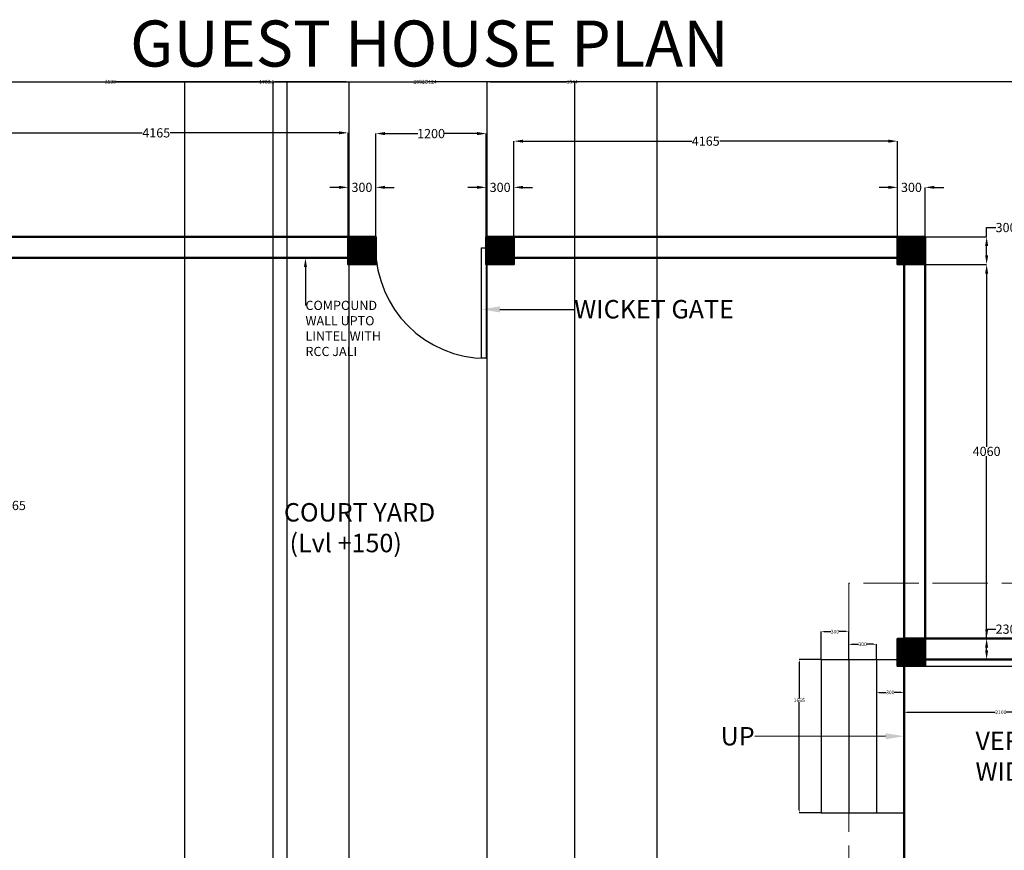
# Model space of a CAD drawing. Units: millimetres. Extents: x -17156 to 39375, y -45872 to -24892.
# Tile 9 of 12: x -5337 to 5351, y -33909 to -24892. Entities that reach past the tile are written whole.
import ezdxf
from ezdxf import colors
from ezdxf.entities.mleader import LeaderData, LeaderLine
from ezdxf.math import Vec2, Vec3

# ---------------------------------------------------------------- set-up
doc = ezdxf.new("R2010")
doc.units = ezdxf.units.MM
doc.header["$MEASUREMENT"] = 0
doc.linetypes.add('ACAD_ISO02W100', pattern=[15, 12, -3])
for name, color, linetype, lineweight in [('A-ANNO-DIMS', 2, 'Continuous', 18), ('A-ANNO-TEXT', 4, 'Continuous', 18), ('A-ANNO-TITL', 4, 'Continuous', 35), ('A-AREA-IDEN', 4, 'Continuous', 25), ('A-COLS', 7, 'Continuous', 40), ('A-ROOF', 8, 'Continuous', 18), ('A-ROOF-OVHD', 8, 'ACAD_ISO02W100', 18), ('DOORS', 6, 'Continuous', 25), ('STEPS', 2, 'Continuous', 25), ('WALLS', 5, 'Continuous', 50)]:
    doc.layers.add(name, color=color, linetype=linetype, lineweight=lineweight)
doc.styles.get("Standard").update_dxf_attribs({"font": 'arial.ttf'})
doc.dimstyles.get("Standard").update_dxf_attribs({"dimtxt": 40, "dimasz": 30.18, "dimexe": 0, "dimexo": 0.0625, "dimgap": 0.09, "dimtad": 0, "dimtih": 1, "dimtoh": 1, "dimdec": 0, "dimzin": 0, "dimdsep": 46, "dimtxsty": 'Standard', "dimcen": 0.09, "dimadec": 0, "dimazin": 0, "dimtfac": 1, "dimtdec": 0, "dimtofl": 0, "dimtmove": 0, "dimatfit": 3, "dimfxl": 1, "dimtolj": 1, "dimtzin": 0, "dimarcsym": 0})

# ---------------------------------------------------------------- blocks, each defined once
blk = doc.blocks.new('*U4')
for p, q in [((-1000, 0), (-1000, 100)), ((0, 0), (0, 100))]:
    blk.add_line(p, q)
blk.add_lwpolyline([(0, 0), (0, -1000), (-43.75, -1000), (-43.75, 0)], close=True)
blk.add_arc((0, 0), 1000, 180, 270)
blk = doc.blocks.new('*D64')
at = {"layer": 'A-ANNO-DIMS', "color": 0, "lineweight": -2, "transparency": 16777216}
for p, q in [((-6272, -31538), (-6272, -30165)), ((-6172, -30165), (-6107, -30165)), ((-6007, -31608), (-6007, -30165)), ((-6007, -30165), (-5496, -30165))]:
    blk.add_line(p, q, dxfattribs=at)
at = {"layer": 'A-ANNO-DIMS', "color": 0, "lineweight": 100, "transparency": 16777216}
for points in [[(-6172, -30148), (-6172, -30181), (-6272, -30165)], [(-6107, -30148), (-6107, -30181), (-6007, -30165)]]:
    blk.add_solid(points, dxfattribs=at)
at = {"layer": 'Defpoints', "color": 0, "lineweight": 100, "transparency": 16777216}
for p in [(-6007, -30165), (-6272, -31538), (-6007, -31608)]:
    blk.add_point(p, dxfattribs=at)
at = {"layer": 'A-ANNO-DIMS', "color": 0, "transparency": 16777216, "insert": (-5384, -30165), "char_height": 100, "attachment_point": 5}
blk.add_mtext('\\A1;265', dxfattribs=at)
blk = doc.blocks.new('*D67')
at = {"layer": 'A-ANNO-DIMS', "color": 0, "lineweight": -2, "transparency": 16777216}
for p, q in [((-5937, -27248), (-5937, -26120)), ((-5837, -26120), (-4007, -26120)), ((-1872, -26120), (-3703, -26120)), ((-1772, -27248), (-1772, -26120))]:
    blk.add_line(p, q, dxfattribs=at)
at = {"layer": 'A-ANNO-DIMS', "color": 0, "lineweight": 100, "transparency": 16777216}
for points in [[(-5837, -26103), (-5837, -26136), (-5937, -26120)], [(-1872, -26103), (-1872, -26136), (-1772, -26120)]]:
    blk.add_solid(points, dxfattribs=at)
at = {"layer": 'Defpoints', "color": 0, "lineweight": 100, "transparency": 16777216}
for p in [(-1772, -26120), (-5937, -27248), (-1772, -27248)]:
    blk.add_point(p, dxfattribs=at)
at = {"layer": 'A-ANNO-DIMS', "color": 0, "transparency": 16777216, "insert": (-3855, -26120), "char_height": 100, "attachment_point": 5}
blk.add_mtext('\\A1;4165', dxfattribs=at)
blk = doc.blocks.new('*D68')
at = {"layer": 'A-ANNO-DIMS', "color": 0, "lineweight": -2, "transparency": 16777216}
for p, q in [((-1872, -26712), (-1972, -26712)), ((-1772, -27248), (-1772, -26712)), ((-1472, -27248), (-1472, -26712)), ((-1372, -26712), (-1272, -26712))]:
    blk.add_line(p, q, dxfattribs=at)
at = {"layer": 'A-ANNO-DIMS', "color": 0, "lineweight": 100, "transparency": 16777216}
for points in [[(-1872, -26695), (-1872, -26728), (-1772, -26712)], [(-1372, -26695), (-1372, -26728), (-1472, -26712)]]:
    blk.add_solid(points, dxfattribs=at)
at = {"layer": 'Defpoints', "color": 0, "lineweight": 100, "transparency": 16777216}
for p in [(-1472, -26712), (-1772, -27248), (-1472, -27248)]:
    blk.add_point(p, dxfattribs=at)
at = {"layer": 'A-ANNO-DIMS', "color": 0, "transparency": 16777216, "insert": (-1622, -26712), "char_height": 100, "attachment_point": 5}
blk.add_mtext('\\A1;300', dxfattribs=at)
blk = doc.blocks.new('*D69')
at = {"layer": 'A-ANNO-DIMS', "color": 0, "lineweight": -2, "transparency": 16777216}
for p, q in [((-1472, -27248), (-1472, -26128)), ((-1372, -26128), (-1017, -26128)), ((-372, -26128), (-728, -26128)), ((-272, -27248), (-272, -26128))]:
    blk.add_line(p, q, dxfattribs=at)
at = {"layer": 'A-ANNO-DIMS', "color": 0, "lineweight": 100, "transparency": 16777216}
for points in [[(-1372, -26111), (-1372, -26145), (-1472, -26128)], [(-372, -26111), (-372, -26145), (-272, -26128)]]:
    blk.add_solid(points, dxfattribs=at)
at = {"layer": 'Defpoints', "color": 0, "lineweight": 100, "transparency": 16777216}
for p in [(-272, -26128), (-1472, -27248), (-272, -27248)]:
    blk.add_point(p, dxfattribs=at)
at = {"layer": 'A-ANNO-DIMS', "color": 0, "transparency": 16777216, "insert": (-872, -26128), "char_height": 100, "attachment_point": 5}
blk.add_mtext('\\A1;1200', dxfattribs=at)
blk = doc.blocks.new('*D70')
at = {"layer": 'A-ANNO-DIMS', "color": 0, "lineweight": -2, "transparency": 16777216}
for p, q in [((-372, -26712), (-472, -26712)), ((-272, -27248), (-272, -26712)), ((28, -27248), (28, -26712)), ((128, -26712), (228, -26712))]:
    blk.add_line(p, q, dxfattribs=at)
at = {"layer": 'A-ANNO-DIMS', "color": 0, "lineweight": 100, "transparency": 16777216}
for points in [[(-372, -26695), (-372, -26728), (-272, -26712)], [(128, -26695), (128, -26728), (28, -26712)]]:
    blk.add_solid(points, dxfattribs=at)
at = {"layer": 'Defpoints', "color": 0, "lineweight": 100, "transparency": 16777216}
for p in [(28, -26712), (-272, -27248), (28, -27248)]:
    blk.add_point(p, dxfattribs=at)
at = {"layer": 'A-ANNO-DIMS', "color": 0, "transparency": 16777216, "insert": (-122, -26712), "char_height": 100, "attachment_point": 5}
blk.add_mtext('\\A1;300', dxfattribs=at)
blk = doc.blocks.new('*D71')
at = {"layer": 'A-ANNO-DIMS', "color": 0, "lineweight": -2, "transparency": 16777216}
for p, q in [((28, -27248), (28, -26210)), ((128, -26210), (1958, -26210)), ((4093, -26210), (2262, -26210)), ((4193, -27248), (4193, -26210))]:
    blk.add_line(p, q, dxfattribs=at)
at = {"layer": 'A-ANNO-DIMS', "color": 0, "lineweight": 100, "transparency": 16777216}
for points in [[(128, -26194), (128, -26227), (28, -26210)], [(4093, -26194), (4093, -26227), (4193, -26210)]]:
    blk.add_solid(points, dxfattribs=at)
at = {"layer": 'Defpoints', "color": 0, "lineweight": 100, "transparency": 16777216}
for p in [(4193, -26210), (28, -27248), (4193, -27248)]:
    blk.add_point(p, dxfattribs=at)
at = {"layer": 'A-ANNO-DIMS', "color": 0, "transparency": 16777216, "insert": (2110, -26210), "char_height": 100, "attachment_point": 5}
blk.add_mtext('\\A1;4165', dxfattribs=at)
blk = doc.blocks.new('*D72')
at = {"layer": 'A-ANNO-DIMS', "color": 0, "lineweight": -2, "transparency": 16777216}
for p, q in [((4093, -26712), (3993, -26712)), ((4193, -27248), (4193, -26712)), ((4493, -27248), (4493, -26712)), ((4593, -26712), (4693, -26712))]:
    blk.add_line(p, q, dxfattribs=at)
at = {"layer": 'A-ANNO-DIMS', "color": 0, "lineweight": 100, "transparency": 16777216}
for points in [[(4093, -26695), (4093, -26728), (4193, -26712)], [(4593, -26695), (4593, -26728), (4493, -26712)]]:
    blk.add_solid(points, dxfattribs=at)
at = {"layer": 'Defpoints', "color": 0, "lineweight": 100, "transparency": 16777216}
for p in [(4493, -26712), (4193, -27248), (4493, -27248)]:
    blk.add_point(p, dxfattribs=at)
at = {"layer": 'A-ANNO-DIMS', "color": 0, "transparency": 16777216, "insert": (4343, -26712), "char_height": 100, "attachment_point": 5}
blk.add_mtext('\\A1;300', dxfattribs=at)
blk = doc.blocks.new('*D73')
at = {"layer": 'A-ANNO-DIMS', "color": 0, "lineweight": -2, "transparency": 16777216}
for p, q in [((5846, -31738), (5846, -31438)), ((5846, -31438), (5946, -31438)), ((4493, -31838), (5846, -31838)), ((4493, -31908), (5846, -31908)), ((5846, -32008), (5846, -32108))]:
    blk.add_line(p, q, dxfattribs=at)
at = {"layer": 'A-ANNO-DIMS', "color": 0, "lineweight": 100, "transparency": 16777216}
for points in [[(5830, -31738), (5863, -31738), (5846, -31838)], [(5830, -32008), (5863, -32008), (5846, -31908)]]:
    blk.add_solid(points, dxfattribs=at)
at = {"layer": 'Defpoints', "color": 0, "lineweight": 100, "transparency": 16777216}
for p in [(4493, -31838), (5846, -31838), (4493, -31908)]:
    blk.add_point(p, dxfattribs=at)
at = {"layer": 'A-ANNO-DIMS', "color": 0, "transparency": 16777216, "insert": (6017, -31438), "char_height": 100, "attachment_point": 5}
blk.add_mtext('\\A1;70', dxfattribs=at)
blk = doc.blocks.new('*D74')
at = {"layer": 'A-ANNO-DIMS', "color": 0, "lineweight": -2, "transparency": 16777216}
for p, q in [((5159, -31608), (5159, -31508)), ((5159, -31508), (5259, -31508)), ((4493, -31608), (5159, -31608)), ((5159, -31738), (5159, -31708)), ((4493, -31838), (5159, -31838))]:
    blk.add_line(p, q, dxfattribs=at)
at = {"layer": 'A-ANNO-DIMS', "color": 0, "lineweight": 100, "transparency": 16777216}
for points in [[(5143, -31708), (5176, -31708), (5159, -31608)], [(5143, -31738), (5176, -31738), (5159, -31838)]]:
    blk.add_solid(points, dxfattribs=at)
at = {"layer": 'Defpoints', "color": 0, "lineweight": 100, "transparency": 16777216}
for p in [(4493, -31608), (5159, -31608), (4493, -31838)]:
    blk.add_point(p, dxfattribs=at)
at = {"layer": 'A-ANNO-DIMS', "color": 0, "transparency": 16777216, "insert": (5370, -31508), "char_height": 100, "attachment_point": 5}
blk.add_mtext('\\A1;230', dxfattribs=at)
blk = doc.blocks.new('*D75')
at = {"layer": 'A-ANNO-DIMS', "color": 0, "lineweight": -2, "transparency": 16777216}
for p, q in [((4493, -27548), (5159, -27548)), ((5159, -27648), (5159, -29527)), ((5159, -31508), (5159, -29629)), ((4493, -31608), (5159, -31608))]:
    blk.add_line(p, q, dxfattribs=at)
at = {"layer": 'A-ANNO-DIMS', "color": 0, "lineweight": 100, "transparency": 16777216}
for points in [[(5143, -27648), (5176, -27648), (5159, -27548)], [(5143, -31508), (5176, -31508), (5159, -31608)]]:
    blk.add_solid(points, dxfattribs=at)
at = {"layer": 'Defpoints', "color": 0, "lineweight": 100, "transparency": 16777216}
for p in [(4493, -27548), (5159, -27548), (4493, -31608)]:
    blk.add_point(p, dxfattribs=at)
at = {"layer": 'A-ANNO-DIMS', "color": 0, "transparency": 16777216, "insert": (5159, -29578), "char_height": 100, "attachment_point": 5}
blk.add_mtext('\\A1;4060', dxfattribs=at)
blk = doc.blocks.new('*D76')
at = {"layer": 'A-ANNO-DIMS', "color": 0, "lineweight": -2, "transparency": 16777216}
for p, q in [((5159, -27248), (5159, -27148)), ((5159, -27148), (5259, -27148)), ((4493, -27248), (5159, -27248)), ((5159, -27448), (5159, -27348)), ((4493, -27548), (5159, -27548))]:
    blk.add_line(p, q, dxfattribs=at)
at = {"layer": 'A-ANNO-DIMS', "color": 0, "lineweight": 100, "transparency": 16777216}
for points in [[(5143, -27348), (5176, -27348), (5159, -27248)], [(5143, -27448), (5176, -27448), (5159, -27548)]]:
    blk.add_solid(points, dxfattribs=at)
at = {"layer": 'Defpoints', "color": 0, "lineweight": 100, "transparency": 16777216}
for p in [(4493, -27248), (5159, -27248), (4493, -27548)]:
    blk.add_point(p, dxfattribs=at)
at = {"layer": 'A-ANNO-DIMS', "color": 0, "transparency": 16777216, "insert": (5370, -27148), "char_height": 100, "attachment_point": 5}
blk.add_mtext('\\A1;300', dxfattribs=at)
blk = doc.blocks.new('*D103')
at = {"layer": 'A-ANNO-DIMS', "color": 0, "lineweight": -2, "transparency": 16777216}
for p, q in [((3363, -31838), (3363, -31535)), ((3393, -31535), (3468, -31535)), ((3632, -31535), (3557, -31535)), ((3663, -31838), (3663, -31535))]:
    blk.add_line(p, q, dxfattribs=at)
at = {"layer": 'A-ANNO-DIMS', "color": 0, "lineweight": 100, "transparency": 16777216}
for points in [[(3393, -31530), (3393, -31540), (3363, -31535)], [(3632, -31530), (3632, -31540), (3663, -31535)]]:
    blk.add_solid(points, dxfattribs=at)
at = {"layer": 'Defpoints', "color": 0, "lineweight": 100, "transparency": 16777216}
for p in [(3663, -31535), (3363, -31838), (3663, -31838)]:
    blk.add_point(p, dxfattribs=at)
at = {"layer": 'A-ANNO-DIMS', "color": 0, "transparency": 16777216, "insert": (3513, -31535), "char_height": 40, "attachment_point": 5}
blk.add_mtext('\\A1;300', dxfattribs=at)
blk = doc.blocks.new('*D104')
at = {"layer": 'A-ANNO-DIMS', "color": 0, "lineweight": -2, "transparency": 16777216}
for p, q in [((3663, -31838), (3663, -31672)), ((3693, -31672), (3768, -31672)), ((3932, -31672), (3857, -31672)), ((3963, -31838), (3963, -31672))]:
    blk.add_line(p, q, dxfattribs=at)
at = {"layer": 'A-ANNO-DIMS', "color": 0, "lineweight": 100, "transparency": 16777216}
for points in [[(3693, -31667), (3693, -31677), (3663, -31672)], [(3932, -31667), (3932, -31677), (3963, -31672)]]:
    blk.add_solid(points, dxfattribs=at)
at = {"layer": 'Defpoints', "color": 0, "lineweight": 100, "transparency": 16777216}
for p in [(3963, -31672), (3663, -31838), (3963, -31838)]:
    blk.add_point(p, dxfattribs=at)
at = {"layer": 'A-ANNO-DIMS', "color": 0, "transparency": 16777216, "insert": (3813, -31672), "char_height": 40, "attachment_point": 5}
blk.add_mtext('\\A1;300', dxfattribs=at)
blk = doc.blocks.new('*D105')
at = {"layer": 'A-ANNO-DIMS', "color": 0, "lineweight": -2, "transparency": 16777216}
for p, q in [((3963, -32194), (3963, -32194)), ((3993, -32194), (4068, -32194)), ((4232, -32194), (4157, -32194)), ((4263, -32194), (4263, -32194))]:
    blk.add_line(p, q, dxfattribs=at)
at = {"layer": 'A-ANNO-DIMS', "color": 0, "lineweight": 100, "transparency": 16777216}
for points in [[(3993, -32189), (3993, -32199), (3963, -32194)], [(4232, -32189), (4232, -32199), (4263, -32194)]]:
    blk.add_solid(points, dxfattribs=at)
at = {"layer": 'Defpoints', "color": 0, "lineweight": 100, "transparency": 16777216}
for p in [(3963, -32194), (4263, -32194), (4263, -32194)]:
    blk.add_point(p, dxfattribs=at)
at = {"layer": 'A-ANNO-DIMS', "color": 0, "transparency": 16777216, "insert": (4113, -32194), "char_height": 40, "attachment_point": 5}
blk.add_mtext('\\A1;300', dxfattribs=at)
blk = doc.blocks.new('*D106')
at = {"layer": 'A-ANNO-DIMS', "color": 0, "lineweight": -2, "transparency": 16777216}
for p, q in [((3363, -31838), (3125, -31838)), ((3125, -31868), (3125, -32259)), ((3125, -33473), (3125, -32300)), ((3363, -33503), (3125, -33503))]:
    blk.add_line(p, q, dxfattribs=at)
at = {"layer": 'A-ANNO-DIMS', "color": 0, "lineweight": 100, "transparency": 16777216}
for points in [[(3120, -31868), (3130, -31868), (3125, -31838)], [(3120, -33473), (3130, -33473), (3125, -33503)]]:
    blk.add_solid(points, dxfattribs=at)
at = {"layer": 'Defpoints', "color": 0, "lineweight": 100, "transparency": 16777216}
for p in [(3363, -31838), (3125, -33503), (3363, -33503)]:
    blk.add_point(p, dxfattribs=at)
at = {"layer": 'A-ANNO-DIMS', "color": 0, "transparency": 16777216, "insert": (3125, -32280), "char_height": 40, "attachment_point": 5}
blk.add_mtext('\\A1;1665', dxfattribs=at)
blk = doc.blocks.new('*D107')
at = {"layer": 'A-ANNO-DIMS', "color": 0, "lineweight": -2, "transparency": 16777216}
for p, q in [((4263, -31890), (4263, -32410)), ((6363, -31890), (6363, -32410)), ((4293, -32410), (5253, -32410)), ((6332, -32410), (5373, -32410))]:
    blk.add_line(p, q, dxfattribs=at)
at = {"layer": 'A-ANNO-DIMS', "color": 0, "lineweight": 100, "transparency": 16777216}
for points in [[(4293, -32405), (4293, -32415), (4263, -32410)], [(6332, -32405), (6332, -32415), (6363, -32410)]]:
    blk.add_solid(points, dxfattribs=at)
at = {"layer": 'Defpoints', "color": 0, "lineweight": 100, "transparency": 16777216}
for p in [(4263, -31890), (6363, -31890), (6363, -32410)]:
    blk.add_point(p, dxfattribs=at)
at = {"layer": 'A-ANNO-DIMS', "color": 0, "transparency": 16777216, "insert": (5313, -32410), "char_height": 40, "attachment_point": 5}
blk.add_mtext('\\A1;2100', dxfattribs=at)
blk = doc.blocks.new('COL-300x300')
h = blk.add_hatch()
h.set_pattern_fill('ANSI31', color=256)
h.paths.add_polyline_path([(300, 300), (0, 300), (0, 0), (300, 0)])
blk.add_lwpolyline([(0, 300), (300, 300), (300, 0), (0, 0)], close=True)
blk = doc.blocks.new('*D144')
at = {"layer": 'A-ANNO-DIMS', "color": 0, "lineweight": -2, "transparency": 16777216}
for p, q in [((-15397, -31008), (-15397, -25565)), ((-15367, -25565), (-1063, -25565)), ((13392, -25565), (-912, -25565)), ((13423, -31008), (13423, -25565))]:
    blk.add_line(p, q, dxfattribs=at)
at = {"layer": 'A-ANNO-DIMS', "color": 0, "lineweight": 100, "transparency": 16777216}
for points in [[(-15367, -25560), (-15367, -25570), (-15397, -25565)], [(13392, -25560), (13392, -25570), (13423, -25565)]]:
    blk.add_solid(points, dxfattribs=at)
at = {"layer": 'Defpoints', "color": 0, "lineweight": 100, "transparency": 16777216}
for p in [(13423, -25565), (-15397, -31008), (13423, -31008)]:
    blk.add_point(p, dxfattribs=at)
at = {"layer": 'A-ANNO-DIMS', "color": 0, "transparency": 16777216, "insert": (-987, -25565), "char_height": 40, "attachment_point": 5}
blk.add_mtext('\\A1;28820', dxfattribs=at)
blk = doc.blocks.new('*D145')
at = {"layer": 'A-ANNO-DIMS', "color": 0, "lineweight": -2, "transparency": 16777216}
for p, q in [((-6237, -27248), (-17080, -27248)), ((-17080, -27278), (-17080, -35685)), ((-17080, -44133), (-17080, -35726)), ((-2887, -44163), (-17080, -44163))]:
    blk.add_line(p, q, dxfattribs=at)
at = {"layer": 'A-ANNO-DIMS', "color": 0, "lineweight": 100, "transparency": 16777216}
for points in [[(-17085, -27278), (-17075, -27278), (-17080, -27248)], [(-17085, -44133), (-17075, -44133), (-17080, -44163)]]:
    blk.add_solid(points, dxfattribs=at)
at = {"layer": 'Defpoints', "color": 0, "lineweight": 100, "transparency": 16777216}
for p in [(-6237, -27248), (-17080, -44163), (-2887, -44163)]:
    blk.add_point(p, dxfattribs=at)
at = {"layer": 'A-ANNO-DIMS', "color": 0, "transparency": 16777216, "insert": (-17080, -35705), "char_height": 40, "attachment_point": 5}
blk.add_mtext('\\A1;16915', dxfattribs=at)
blk = doc.blocks.new('*D148')
at = {"layer": 'A-ANNO-DIMS', "color": 0, "lineweight": -2, "transparency": 16777216}
for p, q in [((-3546, -34838), (-3546, -25565)), ((-3516, -25565), (-2735, -25565)), ((-1792, -25565), (-2573, -25565)), ((-1762, -34838), (-1762, -25565))]:
    blk.add_line(p, q, dxfattribs=at)
at = {"layer": 'A-ANNO-DIMS', "color": 0, "lineweight": 100, "transparency": 16777216}
for points in [[(-3516, -25560), (-3516, -25570), (-3546, -25565)], [(-1792, -25560), (-1792, -25570), (-1762, -25565)]]:
    blk.add_solid(points, dxfattribs=at)
at = {"layer": 'Defpoints', "color": 0, "lineweight": 100, "transparency": 16777216}
for p in [(-1762, -25565), (-3546, -34838), (-1762, -34838)]:
    blk.add_point(p, dxfattribs=at)
at = {"layer": 'A-ANNO-DIMS', "color": 0, "transparency": 16777216, "insert": (-2654, -25565), "char_height": 40, "attachment_point": 5}
blk.add_mtext('\\A1;1783.5', dxfattribs=at)
blk = doc.blocks.new('*D149')
at = {"layer": 'A-ANNO-DIMS', "color": 0, "lineweight": -2, "transparency": 16777216}
for p, q in [((-262, -34838), (-262, -25565)), ((-232, -25565), (602, -25565)), ((1552, -25565), (718, -25565)), ((1582, -34838), (1582, -25565))]:
    blk.add_line(p, q, dxfattribs=at)
at = {"layer": 'A-ANNO-DIMS', "color": 0, "lineweight": 100, "transparency": 16777216}
for points in [[(-232, -25560), (-232, -25570), (-262, -25565)], [(1552, -25560), (1552, -25570), (1582, -25565)]]:
    blk.add_solid(points, dxfattribs=at)
at = {"layer": 'Defpoints', "color": 0, "lineweight": 100, "transparency": 16777216}
for p in [(1582, -25565), (-262, -34838), (1582, -34838)]:
    blk.add_point(p, dxfattribs=at)
at = {"layer": 'A-ANNO-DIMS', "color": 0, "transparency": 16777216, "insert": (660, -25565), "char_height": 40, "attachment_point": 5}
blk.add_mtext('\\A1;1844', dxfattribs=at)
blk = doc.blocks.new('*D151')
at = {"layer": 'A-ANNO-DIMS', "color": 0, "lineweight": -2, "transparency": 16777216}
for p, q in [((-6122, -42548), (-6122, -25565)), ((-6092, -25565), (-4413, -25565)), ((-2615, -25565), (-4294, -25565)), ((-2584, -42548), (-2584, -25565))]:
    blk.add_line(p, q, dxfattribs=at)
at = {"layer": 'A-ANNO-DIMS', "color": 0, "lineweight": 100, "transparency": 16777216}
for points in [[(-6092, -25560), (-6092, -25570), (-6122, -25565)], [(-2615, -25560), (-2615, -25570), (-2584, -25565)]]:
    blk.add_solid(points, dxfattribs=at)
at = {"layer": 'Defpoints', "color": 0, "lineweight": 100, "transparency": 16777216}
for p in [(-2584, -25565), (-6122, -42548), (-2584, -42548)]:
    blk.add_point(p, dxfattribs=at)
at = {"layer": 'A-ANNO-DIMS', "color": 0, "transparency": 16777216, "insert": (-4353, -25565), "char_height": 40, "attachment_point": 5}
blk.add_mtext('\\A1;3538', dxfattribs=at)
blk = doc.blocks.new('*D152')
at = {"layer": 'A-ANNO-DIMS', "color": 0, "lineweight": -2, "transparency": 16777216}
for p, q in [((-2434, -40333), (-2434, -25565)), ((-2404, -25565), (-932, -25565)), ((659, -25565), (-813, -25565)), ((690, -40333), (690, -25565))]:
    blk.add_line(p, q, dxfattribs=at)
at = {"layer": 'A-ANNO-DIMS', "color": 0, "lineweight": 100, "transparency": 16777216}
for points in [[(-2404, -25560), (-2404, -25570), (-2434, -25565)], [(659, -25560), (659, -25570), (690, -25565)]]:
    blk.add_solid(points, dxfattribs=at)
at = {"layer": 'Defpoints', "color": 0, "lineweight": 100, "transparency": 16777216}
for p in [(690, -25565), (-2434, -40333), (690, -40333)]:
    blk.add_point(p, dxfattribs=at)
at = {"layer": 'A-ANNO-DIMS', "color": 0, "transparency": 16777216, "insert": (-872, -25565), "char_height": 40, "attachment_point": 5}
blk.add_mtext('\\A1;3124', dxfattribs=at)

msp = doc.modelspace()

# ---------------------------------------------------------------- linework, layer by layer
at = {"layer": 'A-ROOF'}
msp.add_line((3662.65, -31607.85), (3662.65, -31007.85), dxfattribs=at)
at = {"layer": 'A-ROOF-OVHD', "ltscale": 50}
for p, q in [((13422.65, -31007.85), (3662.65, -31007.85)), ((3662.65, -31607.85), (3662.65, -34237.85))]:
    msp.add_line(p, q, dxfattribs=at)
at = {"layer": 'STEPS'}
for p, q in [((3362.65, -31837.85), (3362.65, -33502.85)), ((3362.65, -31837.85), (4262.65, -31837.85)), ((3662.65, -31837.85), (3662.65, -33502.85)), ((3962.65, -31837.85), (3962.65, -33502.85)), ((3362.65, -33502.85), (4262.65, -33502.85))]:
    msp.add_line(p, q, dxfattribs=at)
at = {"layer": 'WALLS'}
for p, q in [((-6237.35, -27247.85), (-1472.35, -27247.85)), ((-1472.35, -27247.85), (-1472.35, -27477.85)), ((-272.35, -27247.85), (4492.65, -27247.85)), ((4262.65, -27247.85), (4262.65, -31837.85)), ((4492.65, -27247.85), (4492.65, -31837.85)), ((-6237.35, -27477.85), (-1472.35, -27477.85)), ((-272.35, -27477.85), (4492.65, -27477.85)), ((12822.65, -31607.85), (4262.65, -31607.85)), ((4262.65, -31607.85), (4492.65, -31607.85)), ((4262.65, -31607.85), (4262.65, -34837.85)), ((12822.65, -31837.85), (4192.65, -31837.85)), ((4262.65, -31837.85), (4492.65, -31837.85))]:
    msp.add_line(p, q, dxfattribs=at)

# ---------------------------------------------------------------- block references
at = {"layer": 'A-COLS'}
for p in [(-1772.35, -27547.85), (-272.35, -27547.85), (4192.65, -27547.85), (4192.65, -31907.85)]:
    msp.add_blockref('COL-300x300', p, dxfattribs=at)
at = {"layer": 'DOORS', "xscale": 1.2, "yscale": 1.2, "zscale": 1.2}
msp.add_blockref('*U4', (-272.35, -27367.85), dxfattribs=at)

# ---------------------------------------------------------------- texts
at = {"layer": 'A-ANNO-TITL', "insert": (-4138.76, -24900.58), "char_height": 500, "attachment_point": 1}
msp.add_mtext_dynamic_manual_height_columns('{GUEST HOUSE PLAN}', width=17759.1886, gutter_width=1, heights=[0], dxfattribs=at)
at = {"layer": 'A-AREA-IDEN', "char_height": 200, "attachment_point": 1}
for s, width, insert in [('{COURT YARD \\P (Lvl +150)}', 2752.5668, (-2469.03, -30139.46)), ('{VER WIDE}', 660.3665, (5038.26, -32620.61))]:
    msp.add_mtext_dynamic_manual_height_columns(s, width=width, gutter_width=1, heights=[0], dxfattribs=dict(at, insert=insert))

# ---------------------------------------------------------------- dimensions: what is measured, and where the dimension line sits
at = {"layer": 'A-ANNO-DIMS'}
for base, p1, p2, override, picture, middle in [((13422.65, -25564.85), (-15397.35, -31007.85), (13422.65, -31007.85), {"dimdec": 0, "dimlfac": 1, "dimrnd": 0, "dimzin": 0, "dimdsep": 46, "dimlunit": 2}, '*D144', (-987.35, -25564.85)), ((-2584.35, -25564.85), (-6122.35, -42547.85), (-2584.35, -42547.85), {"dimdec": 0, "dimlfac": 1, "dimrnd": 0, "dimzin": 0, "dimdsep": 46, "dimlunit": 2}, '*D151', (-4353.35, -25564.85)), ((-1762.32, -25564.85), (-3545.85, -34837.85), (-1762.32, -34837.85), {"dimdec": 1, "dimlfac": 1, "dimrnd": 0, "dimzin": 0, "dimdsep": 46, "dimlunit": 2}, '*D148', (-2654.08, -25564.85)), ((689.65, -25564.85), (-2434.35, -40332.85), (689.65, -40332.85), {"dimdec": 0, "dimlfac": 1, "dimrnd": 0, "dimzin": 0, "dimdsep": 46, "dimlunit": 2}, '*D152', (-872.35, -25564.85)), ((1581.84, -25564.85), (-262.32, -34837.85), (1581.84, -34837.85), {"dimdec": 0, "dimlfac": 1, "dimrnd": 0, "dimzin": 0, "dimdsep": 46, "dimlunit": 2}, '*D149', (659.76, -25564.85)), ((-272.35, -26127.92), (-1472.35, -27247.85), (-272.35, -27247.85), {"dimtxt": 100, "dimasz": 100, "dimclrd": 0, "dimclre": 0, "dimclrt": 0}, '*D69', (-872.35, -26127.92)), ((-1472.35, -26711.58), (-1772.35, -27247.85), (-1472.35, -27247.85), {"dimtxt": 100, "dimasz": 100, "dimclrd": 0, "dimclre": 0, "dimclrt": 0}, '*D68', (-1622.35, -26711.58)), ((27.65, -26711.58), (-272.35, -27247.85), (27.65, -27247.85), {"dimtxt": 100, "dimasz": 100, "dimclrd": 0, "dimclre": 0, "dimclrt": 0}, '*D70', (-122.35, -26711.58)), ((4492.65, -26711.58), (4192.65, -27247.85), (4492.65, -27247.85), {"dimtxt": 100, "dimasz": 100, "dimclrd": 0, "dimclre": 0, "dimclrt": 0}, '*D72', (4342.65, -26711.58)), ((3662.65, -31535.38), (3362.65, -31837.85), (3662.65, -31837.85), {"dimclrd": 0, "dimclre": 0, "dimclrt": 0}, '*D103', (3512.65, -31535.38)), ((3962.65, -31671.63), (3662.65, -31837.85), (3962.65, -31837.85), {"dimclrd": 0, "dimclre": 0, "dimclrt": 0}, '*D104', (3812.65, -31671.63)), ((4262.65, -32193.89), (3962.65, -32193.89), (4262.65, -32193.89), {"dimclrd": 0, "dimclre": 0, "dimclrt": 0}, '*D105', (4112.65, -32193.89))]:
    dim = msp.add_linear_dim(base=base, p1=p1, p2=p2, dimstyle='Standard', override=override, dxfattribs=at)
    dim.commit()
    dim.dimension.update_dxf_attribs({"geometry": picture, "text_midpoint": middle})
for base, p1, p2, override, picture, middle in [((-1772.35, -26119.65), (-5937.35, -27247.85), (-1772.35, -27247.85), {"dimtxt": 100, "dimasz": 100, "dimclrd": 0, "dimclre": 0, "dimclrt": 0}, '*D67', (-3854.85, -26119.65)), ((4192.65, -26210.5), (27.65, -27247.85), (4192.65, -27247.85), {"dimtxt": 100, "dimasz": 100, "dimclrd": 0, "dimclre": 0, "dimclrt": 0}, '*D71', (2110.15, -26210.5)), ((-6007.35, -30164.55), (-6272.35, -31537.85), (-6007.35, -31607.85), {"dimtxt": 100, "dimasz": 100, "dimclrd": 0, "dimclre": 0, "dimclrt": 0}, '*D64', (-5383.86, -30164.55)), ((6362.65, -32410.02), (4262.65, -31890.1), (6362.65, -31890.1), {"dimclrd": 0, "dimclre": 0, "dimclrt": 0}, '*D107', (5312.65, -32410.02))]:
    dim = msp.add_linear_dim(base=base, p1=p1, p2=p2, dimstyle='Standard', override=override, dxfattribs=at)
    dim.commit()
    dim.dimension.update_dxf_attribs({"geometry": picture, "text_midpoint": middle, "dimtype": 160})
for base, p1, p2, angle, override, picture, middle in [((5159.25, -27247.85), (4492.65, -27547.85), (4492.65, -27247.85), 270, {"dimtxt": 100, "dimasz": 100, "dimclrd": 0, "dimclre": 0, "dimclrt": 0}, '*D76', (5369.61, -27147.85)), ((-17080.35, -44162.85), (-6237.35, -27247.85), (-2887.35, -44162.85), 90, {"dimdec": 0, "dimlfac": 1, "dimrnd": 0, "dimzin": 0, "dimdsep": 46, "dimlunit": 2}, '*D145', (-17080.35, -35705.35)), ((5159.25, -27547.85), (4492.65, -31607.85), (4492.65, -27547.85), 270, {"dimtxt": 100, "dimasz": 100, "dimclrd": 0, "dimclre": 0, "dimclrt": 0}, '*D75', (5159.25, -29577.85)), ((5159.25, -31607.85), (4492.65, -31837.85), (4492.65, -31607.85), 270, {"dimtxt": 100, "dimasz": 100, "dimclrd": 0, "dimclre": 0, "dimclrt": 0}, '*D74', (5370.49, -31507.85))]:
    dim = msp.add_linear_dim(base=base, p1=p1, p2=p2, angle=angle, dimstyle='Standard', override=override, dxfattribs=at)
    dim.commit()
    dim.dimension.update_dxf_attribs({"geometry": picture, "text_midpoint": middle})
for base, p1, p2, angle, override, picture, middle in [((5846.23, -31837.85), (4492.65, -31907.85), (4492.65, -31837.85), 270, {"dimtxt": 100, "dimasz": 100, "dimclrd": 0, "dimclre": 0, "dimclrt": 0}, '*D73', (6017.36, -31437.85)), ((3125.31, -33502.85), (3362.65, -31837.85), (3362.65, -33502.85), 90, {"dimclrd": 0, "dimclre": 0, "dimclrt": 0}, '*D106', (3125.31, -32279.79))]:
    dim = msp.add_linear_dim(base=base, p1=p1, p2=p2, angle=angle, dimstyle='Standard', override=override, dxfattribs=at)
    dim.commit()
    dim.dimension.update_dxf_attribs({"geometry": picture, "text_midpoint": middle, "dimtype": 160})

# ---------------------------------------------------------------- leaders
at = {"layer": 'A-ANNO-TEXT'}
ml = msp.add_multileader_mtext('Standard', dxfattribs=at)
ml.set_content('{\\C4;COMPOUND \\PWALL UPTO\\PLINTEL WITH \\PRCC JALI}', color=256)
ml.set_leader_properties()
ml.build(insert=Vec2(0, 0))
ml.multileader.update_dxf_attribs({"dogleg_length": 0.36, "arrow_head_size": 100})
ctx = ml.context
ctx.base_point, ctx.char_height, ctx.arrow_head_size, ctx.landing_gap_size, ctx.plane_origin = Vec3(-2235.18, -27994.01), 100, 100, 0.09, Vec3(-2235.54, -27477.85)
notes = []
notes.append((ctx, [(0, (1, 1, 0), (-2235.54, -27994.01), (1, 0), 0.36, [(0, [(-2235.54, -27477.85)], 0, [])])]))
ctx.mtext.insert, ctx.mtext.flow_direction = Vec3(-2235.09, -27943.16), 5
ml = msp.add_multileader_mtext('Standard', dxfattribs=at)
ml.set_content('{\\C4;WICKET GATE }', color=256)
ml.set_leader_properties()
ml.build(insert=Vec2(0, 0))
ml.multileader.update_dxf_attribs({"dogleg_length": 0.36, "arrow_head_size": 200})
ctx = ml.context
ctx.base_point, ctx.char_height, ctx.arrow_head_size, ctx.landing_gap_size, ctx.plane_origin = Vec3(682, -28036.44), 200, 200, 0.09, Vec3(-324.85, -28036.44)
notes.append((ctx, [(0, (1, 1, 0), (681.64, -28036.44), (1, 0), 0.36, [(0, [(-324.85, -28036.44)], 0, [])])]))
ctx.mtext.insert, ctx.mtext.flow_direction = Vec3(682.09, -27934.73), 5
ml = msp.add_multileader_mtext('Standard', dxfattribs=at)
ml.set_content('{\\C4;UP}', color=256)
ml.set_leader_properties()
ml.build(insert=Vec2(0, 0))
ml.multileader.update_dxf_attribs({"dogleg_length": 0.36, "arrow_head_size": 200})
ctx = ml.context
ctx.base_point, ctx.char_height, ctx.arrow_head_size, ctx.landing_gap_size, ctx.plane_origin = Vec3(2287.01, -32671.92), 200, 200, 0.09, Vec3(4262.65, -32671.92)
ctx.text_align_type = 2
notes.append((ctx, [(0, (1, 1, 0), (2641.58, -32671.92), (-1, 0), 0.36, [(0, [(4262.65, -32670.15)], 0, [])])]))
ctx.mtext.insert, ctx.mtext.alignment, ctx.mtext.flow_direction = Vec3(2641.13, -32570.22), 3, 5
for ctx, leaders in notes:
    for number, flags, end, landing, length, lines in leaders:
        leader = LeaderData()
        leader.index, (leader.has_last_leader_line, leader.has_dogleg_vector, leader.attachment_direction) = number, flags
        leader.last_leader_point, leader.dogleg_vector, leader.dogleg_length = Vec3(end), Vec3(landing), length
        for number, points, colour, breaks in lines:
            line = LeaderLine()
            line.index, line.vertices, line.color, line.breaks = number, Vec3.list(points), colors.encode_raw_color(colour), breaks
            leader.lines.append(line)
        ctx.leaders.append(leader)

doc.saveas('drawing.dxf')
